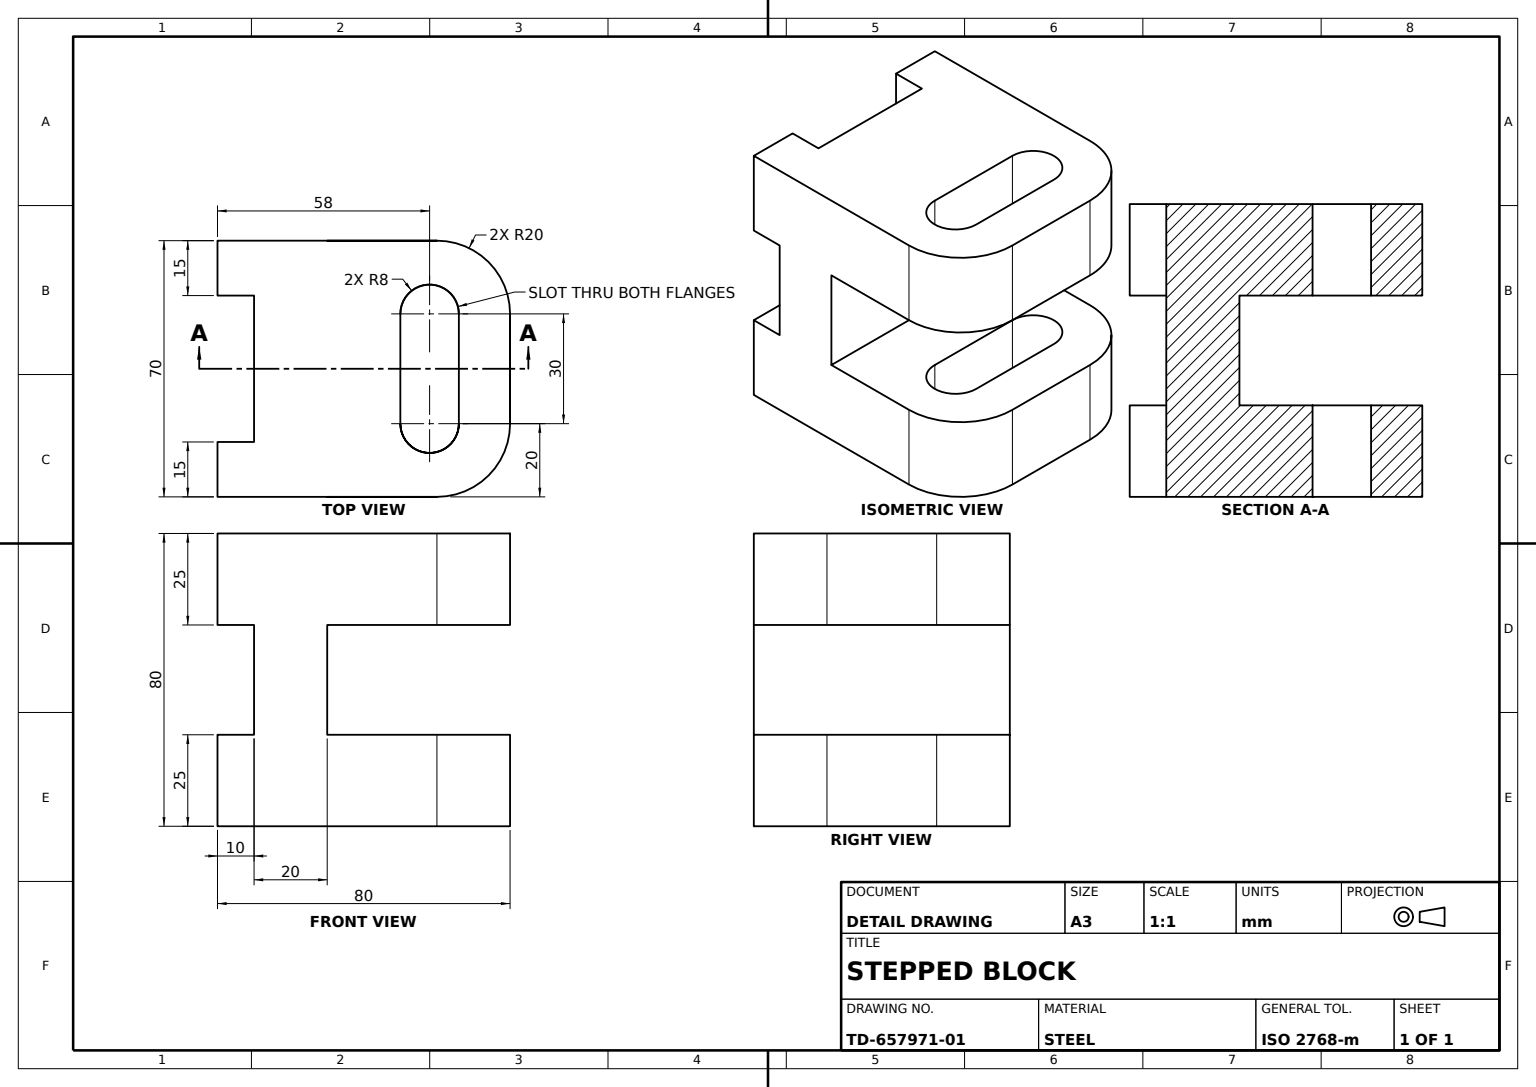
SolidWorks part; units mm, degrees
material "Plain Carbon Steel"
ref_plane "Front Plane" through (0, 0, 0) normal (0, 0, 1) x (1, 0, 0)
ref_plane "Top Plane" through (0, 0, 0) normal (0, 1, 0) x (1, 0, 0)
ref_plane "Right Plane" through (0, 0, 0) normal (1, 0, 0) x (0, 0, -1)
sketch "Base Block Profile" plane through (0, 0, 0) normal (0, 0, 1) x (1, 0, 0)
  line L0 (0, 0) -> (70, 0)
  line L1 (70, 0) -> (70, 80)
  line L2 (70, 80) -> (0, 80)
  line L3 (0, 80) -> (0, 0)
  dimension "D1" = 70
  dimension "D2" = 80
extrude "Base Block 20mm" add sketch "Base Block Profile" along normal blind 20
sketch "H Boss Profile" plane through (0, 0, 20) normal (0, 0, 1) x (1, 0, 0)
  line L0 (0, 80) -> (15, 80)
  line L1 (0, 0) -> (70, 0) construction
  line L2 (0, 80) -> (0, 55)
  line L3 (70, 80) -> (70, 55)
  line L4 (0, 80) -> (0, 0) construction
  line L5 (55, 80) -> (70, 80)
  line L6 (0, 25) -> (0, 0)
  line L7 (70, 80) -> (0, 80) construction
  line L8 (15, 80) -> (15, 55)
  line L9 (15, 55) -> (0, 55)
  line L10 (0, 0) -> (15, 0)
  line L11 (55, 80) -> (55, 55)
  line L12 (55, 55) -> (70, 55)
  line L13 (70, 0) -> (70, 80) construction
  line L14 (0, 25) -> (15, 25)
  line L15 (15, 25) -> (15, 0)
  line L16 (55, 0) -> (55, 25)
  line L17 (55, 25) -> (70, 25)
  line L18 (55, 0) -> (70, 0)
  line L19 (70, 0) -> (70, 25)
  dimension "D1" = 15
  dimension "D2" = 25
extrude "H Boss 10mm" add sketch "H Boss Profile" along normal blind 10
sketch "Rear Boss Profile" plane through (0, 80, 0) normal (0, 1, 0) x (1, 0, 0)
  line L0 (0, 50) -> (70, 50)
  line L2 (0, 50) -> (0, 0)
  line L3 (0, 0) -> (70, 0)
  line L4 (70, 0) -> (70, 50)
  line L6 (70, 0) -> (0, 0) construction
  dimension "D1" = 50
extrude "Rear Boss 25mm" add sketch "Rear Boss Profile" against normal blind 25
sketch "Rear Boss Extension Profile" plane through (0, 0, 0) normal (0, -1, 0) x (1, 0, 0)
  line L0 (0, 0) -> (0, -50)
  line L1 (0, -50) -> (70, -50)
  line L2 (70, -50) -> (70, 0)
  line L3 (70, 0) -> (0, 0)
extrude "Rear Boss Extension 25mm" add sketch "Rear Boss Extension Profile" against normal blind 25
sketch "Slot 8x30 Profile" plane through (0, 0, 0) normal (0, -1, 0) x (1, 0, 0)
  line L0 (0, 30) -> (0, -50) construction
  line L4 (20, -20) -> (50, -20)
  line L5 (20, -36) -> (50, -36)
  arc A0 (20, -20) -> (20, -36) centre (20, -28) ccw
  arc A1 (50, -36) -> (50, -20) centre (50, -28) ccw
  dimension "D1" = 8
  dimension "D3" = 20
  dimension "D2" = 30
  dimension "D4" = 58
extrude "Through Slot 8x30" cut sketch "Slot 8x30 Profile" against normal blind 100
sketch "Lower Notch Profile" plane through (0, 0, 0) normal (0, -1, 0) x (1, 0, 0)
  line L0 (0, -50) -> (0, -30)
  line L1 (0, 30) -> (0, -50) construction
  line L2 (70, -50) -> (70, -30)
  line L3 (0, -50) -> (20, -50)
  line L4 (70, 30) -> (70, -50) construction
  line L6 (50, -50) -> (70, -50)
  arc A0 (0, -30) -> (20, -50) centre (20, -30) ccw
  arc A1 (50, -50) -> (70, -30) centre (50, -30) ccw
  dimension "D1" = 20
extrude "Lower Notch Cut" cut sketch "Lower Notch Profile" against normal blind 100
